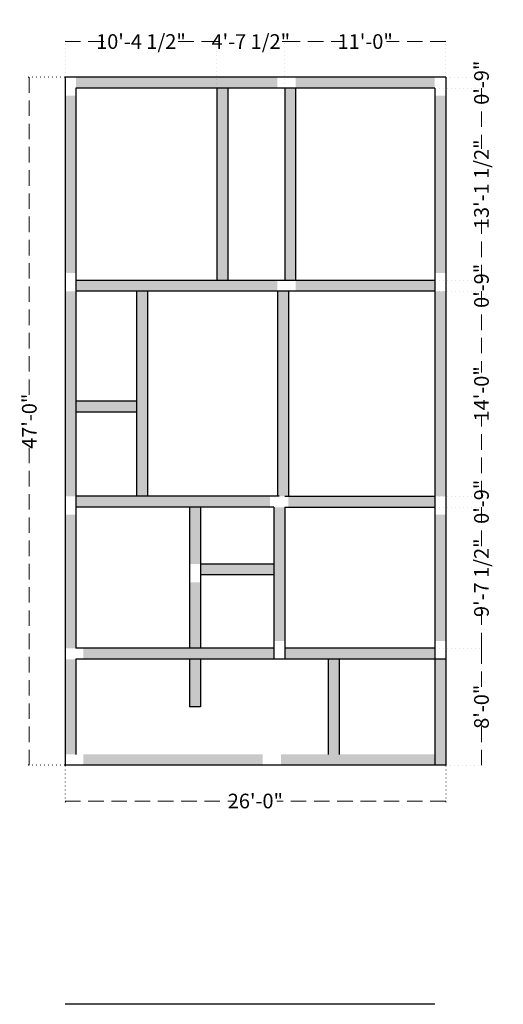
# Model space of a CAD drawing. Units: inches. Extents: x -16911 to -9621, y -48626 to -46270.
# Tile 20 of 20: x -10017 to -9621, y -47224 to -46417. Entities that reach past the tile are written whole.
import ezdxf

# ---------------------------------------------------------------- set-up
doc = ezdxf.new("R2010")
doc.units = ezdxf.units.IN
doc.linetypes.add('DASHED', pattern=[19.05, 12.7, -6.35])
doc.linetypes.add('DOT2', pattern=[3.175, 0, -3.175])
for name, color, linetype, lineweight in [('A-ANNO-DIMS', 2, 'Continuous', 13), ('S-BEAM', 132, 'Continuous', 25), ('S-BEAM-PATT', 254, 'Continuous', 13)]:
    doc.layers.add(name, color=color, linetype=linetype, lineweight=lineweight)
doc.styles.add('style9', font='swisscl.ttf', dxfattribs={"height": 12})
doc.dimstyles.new('Dim9', dxfattribs={"dimtxt": 10, "dimasz": 0.199219, "dimexe": 1, "dimexo": 0.5, "dimgap": 1, "dimtad": 0, "dimdec": 1, "dimzin": 0, "dimdsep": 46, "dimlunit": 4, "dimtxsty": 'style9', "dimblk": 'ARCHTICK', "dimcen": 0.09, "dimclrd": 256, "dimclrt": 256, "dimadec": 0, "dimazin": 0, "dimtfac": 1, "dimtdec": 1, "dimtix": 1, "dimtofl": 0, "dimtmove": 1, "dimatfit": 3, "dimfxl": 9, "dimtolj": 1, "dimtzin": 0, "dimlwd": -1, "dimarcsym": 0})

# ---------------------------------------------------------------- blocks, each defined once
blk = doc.blocks.new('_ArchTick')
at = {"color": 0, "linetype": 'ByBlock', "const_width": 0.15}
blk.add_lwpolyline([(-0.5, -0.5), (0.5, 0.5)], dxfattribs=at)
blk = doc.blocks.new('*D77')
at = {"layer": 'A-ANNO-DIMS', "color": 0, "linetype": 'DOT2', "lineweight": -2, "transparency": 16777216}
for p, q in [((-9979.66, -47028.69), (-9979.66, -47058.44)), ((-9667.66, -47028.69), (-9667.66, -47058.44))]:
    blk.add_line(p, q, dxfattribs=at)
at = {"layer": 'A-ANNO-DIMS', "linetype": 'DASHED', "transparency": 16777216}
for p, q in [((-9979.66, -47057.44), (-9841.21, -47057.44)), ((-9667.66, -47057.44), (-9806.1, -47057.44))]:
    blk.add_line(p, q, dxfattribs=at)
at = {"layer": 'Defpoints', "color": 0, "transparency": 16777216}
for p in [(-9979.66, -47028.19), (-9667.66, -47028.19), (-9667.66, -47057.44)]:
    blk.add_point(p, dxfattribs=at)
at = {"layer": 'A-ANNO-DIMS', "transparency": 16777216, "xscale": 0.19921875, "yscale": 0.19921875, "zscale": 0.19921875, "rotation": 180}
blk.add_blockref('_ArchTick', (-9979.66, -47057.44), dxfattribs=at)
at = {"layer": 'A-ANNO-DIMS', "transparency": 16777216, "xscale": 0.19921875, "yscale": 0.19921875, "zscale": 0.19921875}
blk.add_blockref('_ArchTick', (-9667.66, -47057.44), dxfattribs=at)
at = {"layer": 'A-ANNO-DIMS', "transparency": 16777216, "insert": (-9823.66, -47057.44), "char_height": 12, "attachment_point": 5, "style": 'style9'}
blk.add_mtext('\\A1;26\'-0"', dxfattribs=at)
blk = doc.blocks.new('*D78')
at = {"layer": 'A-ANNO-DIMS', "color": 0, "linetype": 'DOT2', "lineweight": -2, "transparency": 16777216}
for p, q in [((-9980.16, -46464.19), (-10009.91, -46464.19)), ((-9980.16, -47028.19), (-10009.91, -47028.19))]:
    blk.add_line(p, q, dxfattribs=at)
at = {"layer": 'A-ANNO-DIMS', "linetype": 'DASHED', "transparency": 16777216}
for p, q in [((-10008.91, -46464.19), (-10008.91, -46728.55)), ((-10008.91, -47028.19), (-10008.91, -46763.82))]:
    blk.add_line(p, q, dxfattribs=at)
at = {"layer": 'Defpoints', "color": 0, "transparency": 16777216}
for p in [(-9979.66, -46464.19), (-10008.91, -47028.19), (-9979.66, -47028.19)]:
    blk.add_point(p, dxfattribs=at)
at = {"layer": 'A-ANNO-DIMS', "transparency": 16777216, "xscale": 0.19921875, "yscale": 0.19921875, "zscale": 0.19921875}
for p, rotation in [((-10008.91, -46464.19), 90), ((-10008.91, -47028.19), 270)]:
    blk.add_blockref('_ArchTick', p, dxfattribs=dict(at, rotation=rotation))
at = {"layer": 'A-ANNO-DIMS', "transparency": 16777216, "insert": (-10008.91, -46746.19), "char_height": 12, "attachment_point": 5, "rotation": 90, "style": 'style9'}
blk.add_mtext('\\A1;47\'-0"', dxfattribs=at)
blk = doc.blocks.new('*D79')
at = {"layer": 'A-ANNO-DIMS', "color": 0, "linetype": 'DOT2', "lineweight": -2, "transparency": 16777216}
for p, q in [((-9979.66, -46463.69), (-9979.66, -46433.94)), ((-9855.16, -46472.69), (-9855.16, -46433.94))]:
    blk.add_line(p, q, dxfattribs=at)
at = {"layer": 'A-ANNO-DIMS', "linetype": 'DASHED', "transparency": 16777216}
for p, q in [((-9979.66, -46434.94), (-9946.52, -46434.94)), ((-9855.16, -46434.94), (-9888.29, -46434.94))]:
    blk.add_line(p, q, dxfattribs=at)
at = {"layer": 'Defpoints', "color": 0, "transparency": 16777216}
for p in [(-9855.16, -46434.94), (-9979.66, -46464.19), (-9855.16, -46473.19)]:
    blk.add_point(p, dxfattribs=at)
at = {"layer": 'A-ANNO-DIMS', "transparency": 16777216, "xscale": 0.19921875, "yscale": 0.19921875, "zscale": 0.19921875, "rotation": 180}
blk.add_blockref('_ArchTick', (-9979.66, -46434.94), dxfattribs=at)
at = {"layer": 'A-ANNO-DIMS', "transparency": 16777216, "xscale": 0.19921875, "yscale": 0.19921875, "zscale": 0.19921875}
blk.add_blockref('_ArchTick', (-9855.16, -46434.94), dxfattribs=at)
at = {"layer": 'A-ANNO-DIMS', "transparency": 16777216, "insert": (-9917.41, -46434.94), "char_height": 12, "attachment_point": 5, "style": 'style9'}
blk.add_mtext('\\A1;10\'-4 1/2"', dxfattribs=at)
blk = doc.blocks.new('*D80')
at = {"layer": 'A-ANNO-DIMS', "color": 0, "linetype": 'DOT2', "lineweight": -2, "transparency": 16777216}
for p, q in [((-9855.16, -46472.69), (-9855.16, -46433.94)), ((-9799.66, -46472.69), (-9799.66, -46433.94))]:
    blk.add_line(p, q, dxfattribs=at)
at = {"layer": 'A-ANNO-DIMS', "linetype": 'DASHED', "transparency": 16777216}
for p, q in [((-9855.16, -46434.94), (-9852.98, -46434.94)), ((-9799.66, -46434.94), (-9801.83, -46434.94))]:
    blk.add_line(p, q, dxfattribs=at)
at = {"layer": 'Defpoints', "color": 0, "transparency": 16777216}
for p in [(-9799.66, -46434.94), (-9855.16, -46473.19), (-9799.66, -46473.19)]:
    blk.add_point(p, dxfattribs=at)
at = {"layer": 'A-ANNO-DIMS', "transparency": 16777216, "xscale": 0.19921875, "yscale": 0.19921875, "zscale": 0.19921875, "rotation": 180}
blk.add_blockref('_ArchTick', (-9855.16, -46434.94), dxfattribs=at)
at = {"layer": 'A-ANNO-DIMS', "transparency": 16777216, "xscale": 0.19921875, "yscale": 0.19921875, "zscale": 0.19921875}
blk.add_blockref('_ArchTick', (-9799.66, -46434.94), dxfattribs=at)
at = {"layer": 'A-ANNO-DIMS', "transparency": 16777216, "insert": (-9827.41, -46434.94), "char_height": 12, "attachment_point": 5, "style": 'style9'}
blk.add_mtext('\\A1;4\'-7 1/2"', dxfattribs=at)
blk = doc.blocks.new('*D81')
at = {"layer": 'A-ANNO-DIMS', "color": 0, "linetype": 'DOT2', "lineweight": -2, "transparency": 16777216}
for p, q in [((-9799.66, -46472.69), (-9799.66, -46433.94)), ((-9667.66, -46463.69), (-9667.66, -46433.94))]:
    blk.add_line(p, q, dxfattribs=at)
at = {"layer": 'A-ANNO-DIMS', "linetype": 'DASHED', "transparency": 16777216}
for p, q in [((-9799.66, -46434.94), (-9751.08, -46434.94)), ((-9667.66, -46434.94), (-9716.24, -46434.94))]:
    blk.add_line(p, q, dxfattribs=at)
at = {"layer": 'Defpoints', "color": 0, "transparency": 16777216}
for p in [(-9667.66, -46434.94), (-9667.66, -46464.19), (-9799.66, -46473.19)]:
    blk.add_point(p, dxfattribs=at)
at = {"layer": 'A-ANNO-DIMS', "transparency": 16777216, "xscale": 0.19921875, "yscale": 0.19921875, "zscale": 0.19921875, "rotation": 180}
blk.add_blockref('_ArchTick', (-9799.66, -46434.94), dxfattribs=at)
at = {"layer": 'A-ANNO-DIMS', "transparency": 16777216, "xscale": 0.19921875, "yscale": 0.19921875, "zscale": 0.19921875}
blk.add_blockref('_ArchTick', (-9667.66, -46434.94), dxfattribs=at)
at = {"layer": 'A-ANNO-DIMS', "transparency": 16777216, "insert": (-9733.66, -46434.94), "char_height": 12, "attachment_point": 5, "style": 'style9'}
blk.add_mtext('\\A1;11\'-0"', dxfattribs=at)
blk = doc.blocks.new('*D82')
at = {"layer": 'A-ANNO-DIMS', "color": 0, "linetype": 'DOT2', "lineweight": -2, "transparency": 16777216}
for p, q in [((-9667.16, -46464.19), (-9637.41, -46464.19)), ((-9676.16, -46473.19), (-9637.41, -46473.19))]:
    blk.add_line(p, q, dxfattribs=at)
at = {"layer": 'A-ANNO-DIMS', "linetype": 'DASHED', "transparency": 16777216}
for p, q in [((-9638.41, -46464.19), (-9638.41, -46463.99)), ((-9638.41, -46473.19), (-9638.41, -46473.39))]:
    blk.add_line(p, q, dxfattribs=at)
at = {"layer": 'Defpoints', "color": 0, "transparency": 16777216}
for p in [(-9667.66, -46464.19), (-9676.66, -46473.19), (-9638.41, -46473.19)]:
    blk.add_point(p, dxfattribs=at)
at = {"layer": 'A-ANNO-DIMS', "transparency": 16777216, "xscale": 0.19921875, "yscale": 0.19921875, "zscale": 0.19921875}
for p, rotation in [((-9638.41, -46464.19), 270), ((-9638.41, -46473.19), 90)]:
    blk.add_blockref('_ArchTick', p, dxfattribs=dict(at, rotation=rotation))
at = {"layer": 'A-ANNO-DIMS', "transparency": 16777216, "insert": (-9638.41, -46468.69), "char_height": 12, "attachment_point": 5, "rotation": 90, "style": 'style9'}
blk.add_mtext('\\A1;0\'-9"', dxfattribs=at)
blk = doc.blocks.new('*D83')
at = {"layer": 'A-ANNO-DIMS', "color": 0, "linetype": 'DOT2', "lineweight": -2, "transparency": 16777216}
for p, q in [((-9676.16, -46473.19), (-9637.41, -46473.19)), ((-9676.16, -46630.69), (-9637.41, -46630.69))]:
    blk.add_line(p, q, dxfattribs=at)
at = {"layer": 'A-ANNO-DIMS', "linetype": 'DASHED', "transparency": 16777216}
for p, q in [((-9638.41, -46473.19), (-9638.41, -46522.82)), ((-9638.41, -46630.69), (-9638.41, -46581.06))]:
    blk.add_line(p, q, dxfattribs=at)
at = {"layer": 'Defpoints', "color": 0, "transparency": 16777216}
for p in [(-9676.66, -46473.19), (-9676.66, -46630.69), (-9638.41, -46630.69)]:
    blk.add_point(p, dxfattribs=at)
at = {"layer": 'A-ANNO-DIMS', "transparency": 16777216, "xscale": 0.19921875, "yscale": 0.19921875, "zscale": 0.19921875}
for p, rotation in [((-9638.41, -46473.19), 90), ((-9638.41, -46630.69), 270)]:
    blk.add_blockref('_ArchTick', p, dxfattribs=dict(at, rotation=rotation))
at = {"layer": 'A-ANNO-DIMS', "transparency": 16777216, "insert": (-9638.41, -46551.94), "char_height": 12, "attachment_point": 5, "rotation": 90, "style": 'style9'}
blk.add_mtext('\\A1;13\'-1 1/2"', dxfattribs=at)
blk = doc.blocks.new('*D84')
at = {"layer": 'A-ANNO-DIMS', "color": 0, "linetype": 'DOT2', "lineweight": -2, "transparency": 16777216}
for p, q in [((-9676.16, -46630.69), (-9637.41, -46630.69)), ((-9676.16, -46639.69), (-9637.41, -46639.69))]:
    blk.add_line(p, q, dxfattribs=at)
at = {"layer": 'A-ANNO-DIMS', "linetype": 'DASHED', "transparency": 16777216}
for p, q in [((-9638.41, -46630.69), (-9638.41, -46630.49)), ((-9638.41, -46639.69), (-9638.41, -46639.89))]:
    blk.add_line(p, q, dxfattribs=at)
at = {"layer": 'Defpoints', "color": 0, "transparency": 16777216}
for p in [(-9676.66, -46630.69), (-9676.66, -46639.69), (-9638.41, -46639.69)]:
    blk.add_point(p, dxfattribs=at)
at = {"layer": 'A-ANNO-DIMS', "transparency": 16777216, "xscale": 0.19921875, "yscale": 0.19921875, "zscale": 0.19921875}
for p, rotation in [((-9638.41, -46630.69), 270), ((-9638.41, -46639.69), 90)]:
    blk.add_blockref('_ArchTick', p, dxfattribs=dict(at, rotation=rotation))
at = {"layer": 'A-ANNO-DIMS', "transparency": 16777216, "insert": (-9638.41, -46635.19), "char_height": 12, "attachment_point": 5, "rotation": 90, "style": 'style9'}
blk.add_mtext('\\A1;0\'-9"', dxfattribs=at)
blk = doc.blocks.new('*D85')
at = {"layer": 'A-ANNO-DIMS', "color": 0, "linetype": 'DOT2', "lineweight": -2, "transparency": 16777216}
for p, q in [((-9676.16, -46639.69), (-9637.41, -46639.69)), ((-9676.16, -46807.69), (-9637.41, -46807.69))]:
    blk.add_line(p, q, dxfattribs=at)
at = {"layer": 'A-ANNO-DIMS', "linetype": 'DASHED', "transparency": 16777216}
for p, q in [((-9638.41, -46639.69), (-9638.41, -46706.27)), ((-9638.41, -46807.69), (-9638.41, -46741.11))]:
    blk.add_line(p, q, dxfattribs=at)
at = {"layer": 'Defpoints', "color": 0, "transparency": 16777216}
for p in [(-9676.66, -46639.69), (-9676.66, -46807.69), (-9638.41, -46807.69)]:
    blk.add_point(p, dxfattribs=at)
at = {"layer": 'A-ANNO-DIMS', "transparency": 16777216, "xscale": 0.19921875, "yscale": 0.19921875, "zscale": 0.19921875}
for p, rotation in [((-9638.41, -46639.69), 90), ((-9638.41, -46807.69), 270)]:
    blk.add_blockref('_ArchTick', p, dxfattribs=dict(at, rotation=rotation))
at = {"layer": 'A-ANNO-DIMS', "transparency": 16777216, "insert": (-9638.41, -46723.69), "char_height": 12, "attachment_point": 5, "rotation": 90, "style": 'style9'}
blk.add_mtext('\\A1;14\'-0"', dxfattribs=at)
blk = doc.blocks.new('*D86')
at = {"layer": 'A-ANNO-DIMS', "color": 0, "linetype": 'DOT2', "lineweight": -2, "transparency": 16777216}
for p, q in [((-9676.16, -46807.69), (-9637.41, -46807.69)), ((-9676.16, -46816.69), (-9637.41, -46816.69))]:
    blk.add_line(p, q, dxfattribs=at)
at = {"layer": 'A-ANNO-DIMS', "linetype": 'DASHED', "transparency": 16777216}
for p, q in [((-9638.41, -46807.69), (-9638.41, -46807.49)), ((-9638.41, -46816.69), (-9638.41, -46816.89))]:
    blk.add_line(p, q, dxfattribs=at)
at = {"layer": 'Defpoints', "color": 0, "transparency": 16777216}
for p in [(-9676.66, -46807.69), (-9676.66, -46816.69), (-9638.41, -46816.69)]:
    blk.add_point(p, dxfattribs=at)
at = {"layer": 'A-ANNO-DIMS', "transparency": 16777216, "xscale": 0.19921875, "yscale": 0.19921875, "zscale": 0.19921875}
for p, rotation in [((-9638.41, -46807.69), 270), ((-9638.41, -46816.69), 90)]:
    blk.add_blockref('_ArchTick', p, dxfattribs=dict(at, rotation=rotation))
at = {"layer": 'A-ANNO-DIMS', "transparency": 16777216, "insert": (-9638.41, -46812.19), "char_height": 12, "attachment_point": 5, "rotation": 90, "style": 'style9'}
blk.add_mtext('\\A1;0\'-9"', dxfattribs=at)
blk = doc.blocks.new('*D87')
at = {"layer": 'A-ANNO-DIMS', "color": 0, "linetype": 'DOT2', "lineweight": -2, "transparency": 16777216}
for p, q in [((-9676.16, -46816.69), (-9637.41, -46816.69)), ((-9676.16, -46932.19), (-9637.41, -46932.19))]:
    blk.add_line(p, q, dxfattribs=at)
at = {"layer": 'A-ANNO-DIMS', "linetype": 'DASHED', "transparency": 16777216}
for p, q in [((-9638.41, -46816.69), (-9638.41, -46848.92)), ((-9638.41, -46932.19), (-9638.41, -46899.96))]:
    blk.add_line(p, q, dxfattribs=at)
at = {"layer": 'Defpoints', "color": 0, "transparency": 16777216}
for p in [(-9676.66, -46816.69), (-9676.66, -46932.19), (-9638.41, -46932.19)]:
    blk.add_point(p, dxfattribs=at)
at = {"layer": 'A-ANNO-DIMS', "transparency": 16777216, "xscale": 0.19921875, "yscale": 0.19921875, "zscale": 0.19921875}
for p, rotation in [((-9638.41, -46816.69), 90), ((-9638.41, -46932.19), 270)]:
    blk.add_blockref('_ArchTick', p, dxfattribs=dict(at, rotation=rotation))
at = {"layer": 'A-ANNO-DIMS', "transparency": 16777216, "insert": (-9638.41, -46874.44), "char_height": 12, "attachment_point": 5, "rotation": 90, "style": 'style9'}
blk.add_mtext('\\A1;9\'-7 1/2"', dxfattribs=at)
blk = doc.blocks.new('*D88')
at = {"layer": 'A-ANNO-DIMS', "color": 0, "linetype": 'DOT2', "lineweight": -2, "transparency": 16777216}
for p, q in [((-9676.16, -46932.19), (-9637.41, -46932.19)), ((-9667.16, -47028.19), (-9637.41, -47028.19))]:
    blk.add_line(p, q, dxfattribs=at)
at = {"layer": 'A-ANNO-DIMS', "linetype": 'DASHED', "transparency": 16777216}
for p, q in [((-9638.41, -46932.19), (-9638.41, -46966.37)), ((-9638.41, -47028.19), (-9638.41, -46994))]:
    blk.add_line(p, q, dxfattribs=at)
at = {"layer": 'Defpoints', "color": 0, "transparency": 16777216}
for p in [(-9676.66, -46932.19), (-9667.66, -47028.19), (-9638.41, -47028.19)]:
    blk.add_point(p, dxfattribs=at)
at = {"layer": 'A-ANNO-DIMS', "transparency": 16777216, "xscale": 0.19921875, "yscale": 0.19921875, "zscale": 0.19921875}
for p, rotation in [((-9638.41, -46932.19), 90), ((-9638.41, -47028.19), 270)]:
    blk.add_blockref('_ArchTick', p, dxfattribs=dict(at, rotation=rotation))
at = {"layer": 'A-ANNO-DIMS', "transparency": 16777216, "insert": (-9638.41, -46980.19), "char_height": 12, "attachment_point": 5, "rotation": 90, "style": 'style9'}
blk.add_mtext('\\A1;8\'-0"', dxfattribs=at)

msp = doc.modelspace()

# ---------------------------------------------------------------- hatches: boundary and pattern name
at = {"layer": 'S-BEAM-PATT'}
h = msp.add_hatch(color=256, dxfattribs=at)
h.dxf.hatch_style = 1
h.paths.add_polyline_path([(-9805.658, -46464.188), (-9970.658, -46464.188), (-9970.658, -46473.188), (-9805.658, -46473.188)])
h = msp.add_hatch(color=256, dxfattribs=at)
h.dxf.hatch_style = 1
h.paths.add_polyline_path([(-9676.658, -46464.188), (-9790.658, -46464.188), (-9790.658, -46473.188), (-9676.658, -46473.188)])
h = msp.add_hatch(color=256, dxfattribs=at)
h.dxf.hatch_style = 1
h.paths.add_polyline_path([(-9846.158, -46473.188), (-9855.158, -46473.188), (-9855.158, -46630.688), (-9846.158, -46630.688)])
h = msp.add_hatch(color=256, dxfattribs=at)
h.dxf.hatch_style = 1
h.paths.add_polyline_path([(-9790.658, -46473.188), (-9799.658, -46473.188), (-9799.658, -46630.688), (-9790.658, -46630.688)])
h = msp.add_hatch(color=256, dxfattribs=at)
h.dxf.hatch_style = 1
h.paths.add_polyline_path([(-9970.658, -46479.188), (-9979.658, -46479.188), (-9979.658, -46624.688), (-9970.658, -46624.688)])
h = msp.add_hatch(color=256, dxfattribs=at)
h.dxf.hatch_style = 1
h.paths.add_polyline_path([(-9667.658, -46479.188), (-9676.658, -46479.188), (-9676.658, -46624.688), (-9667.658, -46624.688)])
h = msp.add_hatch(color=256, dxfattribs=at)
h.dxf.hatch_style = 1
h.paths.add_polyline_path([(-9805.658, -46630.688), (-9970.658, -46630.688), (-9970.658, -46639.688), (-9805.658, -46639.688)])
h = msp.add_hatch(color=256, dxfattribs=at)
h.dxf.hatch_style = 1
h.paths.add_polyline_path([(-9676.658, -46630.688), (-9790.658, -46630.688), (-9790.658, -46639.688), (-9676.658, -46639.688)])
h = msp.add_hatch(color=256, dxfattribs=at)
h.dxf.hatch_style = 1
h.paths.add_polyline_path([(-9970.658, -46639.688), (-9979.658, -46639.688), (-9979.658, -46807.688), (-9970.658, -46807.688)])
h = msp.add_hatch(color=256, dxfattribs=at)
h.dxf.hatch_style = 1
h.paths.add_polyline_path([(-9912.058, -46639.688), (-9921.058, -46639.688), (-9921.058, -46807.688), (-9912.058, -46807.688)])
h = msp.add_hatch(color=256, dxfattribs=at)
h.dxf.hatch_style = 1
h.paths.add_polyline_path([(-9796.658, -46639.688), (-9805.658, -46639.688), (-9805.658, -46807.688), (-9796.658, -46807.688)])
h = msp.add_hatch(color=256, dxfattribs=at)
h.dxf.hatch_style = 1
h.paths.add_polyline_path([(-9667.658, -46639.688), (-9676.658, -46639.688), (-9676.658, -46807.688), (-9667.658, -46807.688)])
h = msp.add_hatch(color=256, dxfattribs=at)
h.dxf.hatch_style = 1
h.paths.add_polyline_path([(-9921.058, -46729.688), (-9970.658, -46729.688), (-9970.658, -46738.688), (-9921.058, -46738.688)])
h = msp.add_hatch(color=256, dxfattribs=at)
h.dxf.hatch_style = 1
h.paths.add_polyline_path([(-9811.658, -46807.688), (-9970.658, -46807.688), (-9970.658, -46816.688), (-9811.658, -46816.688)])
h = msp.add_hatch(color=256, dxfattribs=at)
h.dxf.hatch_style = 1
h.paths.add_polyline_path([(-9676.658, -46807.688), (-9796.658, -46807.688), (-9796.658, -46816.688), (-9676.658, -46816.688)])
h = msp.add_hatch(color=256, dxfattribs=at)
h.dxf.hatch_style = 1
h.paths.add_polyline_path([(-9970.658, -46822.688), (-9979.658, -46822.688), (-9979.658, -46932.188), (-9970.658, -46932.188)])
h = msp.add_hatch(color=256, dxfattribs=at)
h.dxf.hatch_style = 1
h.paths.add_polyline_path([(-9868.658, -46816.688), (-9877.658, -46816.688), (-9877.658, -46863.188), (-9868.658, -46863.188)])
h = msp.add_hatch(color=256, dxfattribs=at)
h.dxf.hatch_style = 1
h.paths.add_polyline_path([(-9799.658, -46816.688), (-9808.658, -46816.688), (-9808.658, -46926.188), (-9799.658, -46926.188)])
h = msp.add_hatch(color=256, dxfattribs=at)
h.dxf.hatch_style = 1
h.paths.add_polyline_path([(-9667.658, -46822.688), (-9676.658, -46822.688), (-9676.658, -46926.188), (-9667.658, -46926.188)])
h = msp.add_hatch(color=256, dxfattribs=at)
h.dxf.hatch_style = 1
h.paths.add_polyline_path([(-9808.658, -46863.188), (-9868.658, -46863.188), (-9868.658, -46872.188), (-9808.658, -46872.188)])
h = msp.add_hatch(color=256, dxfattribs=at)
h.dxf.hatch_style = 1
h.paths.add_polyline_path([(-9868.658, -46878.188), (-9877.658, -46878.188), (-9877.658, -46932.188), (-9868.658, -46932.188)])
h = msp.add_hatch(color=256, dxfattribs=at)
h.dxf.hatch_style = 1
h.paths.add_polyline_path([(-9808.658, -46932.188), (-9964.658, -46932.188), (-9964.658, -46941.188), (-9808.658, -46941.188)])
h = msp.add_hatch(color=256, dxfattribs=at)
h.dxf.hatch_style = 1
h.paths.add_polyline_path([(-9676.658, -46932.188), (-9799.658, -46932.188), (-9799.658, -46941.188), (-9676.658, -46941.188)])
h = msp.add_hatch(color=256, dxfattribs=at)
h.dxf.hatch_style = 1
h.paths.add_polyline_path([(-9970.658, -46941.188), (-9979.658, -46941.188), (-9979.658, -47019.188), (-9970.658, -47019.188)])
h = msp.add_hatch(color=256, dxfattribs=at)
h.dxf.hatch_style = 1
h.paths.add_polyline_path([(-9868.658, -46941.188), (-9877.658, -46941.188), (-9877.658, -46980.188), (-9868.658, -46980.188)])
h = msp.add_hatch(color=256, dxfattribs=at)
h.dxf.hatch_style = 1
h.paths.add_polyline_path([(-9754.658, -46941.188), (-9763.658, -46941.188), (-9763.658, -47019.188), (-9754.658, -47019.188)])
h = msp.add_hatch(color=256, dxfattribs=at)
h.dxf.hatch_style = 1
h.paths.add_polyline_path([(-9667.658, -46941.188), (-9676.658, -46941.188), (-9676.658, -47028.188), (-9667.658, -47028.188)])
h = msp.add_hatch(color=256, dxfattribs=at)
h.dxf.hatch_style = 1
h.paths.add_polyline_path([(-9817.658, -47019.188), (-9964.658, -47019.188), (-9964.658, -47028.188), (-9817.658, -47028.188)])
h = msp.add_hatch(color=256, dxfattribs=at)
h.dxf.hatch_style = 1
h.paths.add_polyline_path([(-9676.658, -47019.188), (-9802.658, -47019.188), (-9802.658, -47028.188), (-9676.658, -47028.188)])

# ---------------------------------------------------------------- linework, layer by layer
at = {"layer": 'S-BEAM'}
for p, q in [((-9667.658, -46464.188), (-9979.658, -46464.188)), ((-9979.658, -46464.188), (-9979.658, -47028.188)), ((-9667.658, -46464.188), (-9667.658, -47028.188)), ((-9676.658, -46473.188), (-9970.658, -46473.188)), ((-9970.658, -46473.188), (-9970.658, -46932.188)), ((-9855.158, -46473.188), (-9855.158, -46630.688)), ((-9846.158, -46473.188), (-9846.158, -46630.688)), ((-9799.658, -46473.188), (-9799.658, -46630.688)), ((-9790.658, -46473.188), (-9790.658, -46630.688)), ((-9676.658, -46473.188), (-9676.658, -47028.188)), ((-9676.658, -46630.688), (-9970.658, -46630.688)), ((-9676.658, -46639.688), (-9970.658, -46639.688)), ((-9921.058, -46639.688), (-9921.058, -46807.688)), ((-9912.058, -46639.688), (-9912.058, -46807.688)), ((-9805.658, -46639.688), (-9805.658, -46807.688)), ((-9796.658, -46639.688), (-9796.658, -46807.688)), ((-9921.058, -46729.688), (-9970.658, -46729.688)), ((-9921.058, -46738.688), (-9970.658, -46738.688)), ((-9804.158, -46807.688), (-9970.658, -46807.688)), ((-9799.658, -46807.688), (-9676.658, -46807.688)), ((-9808.658, -46816.688), (-9970.658, -46816.688)), ((-9877.658, -46816.688), (-9877.658, -46932.188)), ((-9868.658, -46816.688), (-9868.658, -46932.188)), ((-9808.658, -46816.688), (-9808.658, -46941.188)), ((-9799.658, -46816.688), (-9799.658, -46941.188)), ((-9799.658, -46816.688), (-9676.658, -46816.688)), ((-9808.658, -46863.188), (-9868.658, -46863.188)), ((-9808.658, -46872.188), (-9868.658, -46872.188)), ((-9808.658, -46932.188), (-9970.658, -46932.188)), ((-9676.658, -46932.188), (-9799.658, -46932.188)), ((-9667.658, -46941.188), (-9970.658, -46941.188)), ((-9970.658, -46941.188), (-9970.658, -47019.188)), ((-9877.658, -46941.188), (-9877.658, -46980.188)), ((-9868.658, -46941.188), (-9868.658, -46980.188)), ((-9763.658, -47019.188), (-9763.658, -46941.188)), ((-9754.658, -47019.188), (-9754.658, -46941.188)), ((-9868.658, -46980.188), (-9877.658, -46980.188)), ((-9667.658, -47028.188), (-9979.658, -47028.188)), ((-9676.658, -47224.073), (-9979.658, -47224.073))]:
    msp.add_line(p, q, dxfattribs=at)

# ---------------------------------------------------------------- dimensions: what is measured, and where the dimension line sits
at = {"layer": 'A-ANNO-DIMS'}
for base, p1, p2, picture, middle in [((-9855.158, -46434.938), (-9979.658, -46464.188), (-9855.158, -46473.188), '*D79', (-9917.408, -46434.938)), ((-9799.658, -46434.938), (-9855.158, -46473.188), (-9799.658, -46473.188), '*D80', (-9827.408, -46434.938)), ((-9667.658, -46434.938), (-9799.658, -46473.188), (-9667.658, -46464.188), '*D81', (-9733.658, -46434.938)), ((-9667.658, -47057.438), (-9979.658, -47028.188), (-9667.658, -47028.188), '*D77', (-9823.658, -47057.438))]:
    dim = msp.add_linear_dim(base=base, p1=p1, p2=p2, dimstyle='Dim9', override={"dimdec": 1, "dimlfac": 1, "dimrnd": 0, "dimzin": 1, "dimdsep": 46, "dimlunit": 4, "dimfrac": 2}, dxfattribs=at)
    dim.commit()
    dim.dimension.update_dxf_attribs({"geometry": picture, "text_midpoint": middle})
for base, p1, p2, picture, middle in [((-9638.408, -46473.188), (-9667.658, -46464.188), (-9676.658, -46473.188), '*D82', (-9638.408, -46468.688)), ((-10008.908, -47028.188), (-9979.658, -46464.188), (-9979.658, -47028.188), '*D78', (-10008.908, -46746.188)), ((-9638.408, -46630.688), (-9676.658, -46473.188), (-9676.658, -46630.688), '*D83', (-9638.408, -46551.938)), ((-9638.408, -46639.688), (-9676.658, -46630.688), (-9676.658, -46639.688), '*D84', (-9638.408, -46635.188)), ((-9638.408, -46807.688), (-9676.658, -46639.688), (-9676.658, -46807.688), '*D85', (-9638.408, -46723.688)), ((-9638.408, -46816.688), (-9676.658, -46807.688), (-9676.658, -46816.688), '*D86', (-9638.408, -46812.188)), ((-9638.408, -46932.188), (-9676.658, -46816.688), (-9676.658, -46932.188), '*D87', (-9638.408, -46874.438)), ((-9638.408, -47028.188), (-9676.658, -46932.188), (-9667.658, -47028.188), '*D88', (-9638.408, -46980.188))]:
    dim = msp.add_linear_dim(base=base, p1=p1, p2=p2, angle=90, dimstyle='Dim9', override={"dimdec": 1, "dimlfac": 1, "dimrnd": 0, "dimzin": 1, "dimdsep": 46, "dimlunit": 4, "dimfrac": 2}, dxfattribs=at)
    dim.commit()
    dim.dimension.update_dxf_attribs({"geometry": picture, "text_midpoint": middle})

doc.saveas('drawing.dxf')
